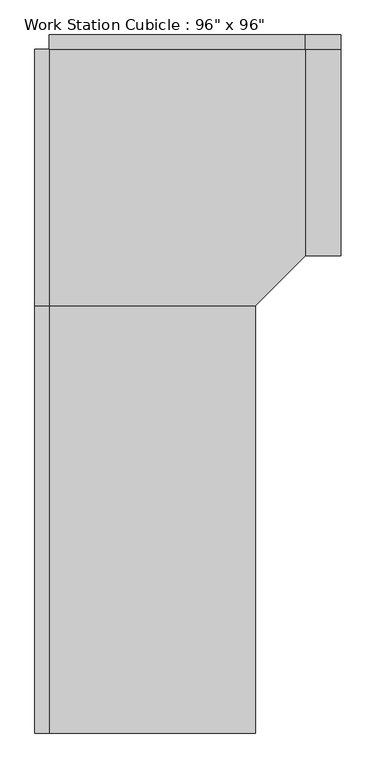
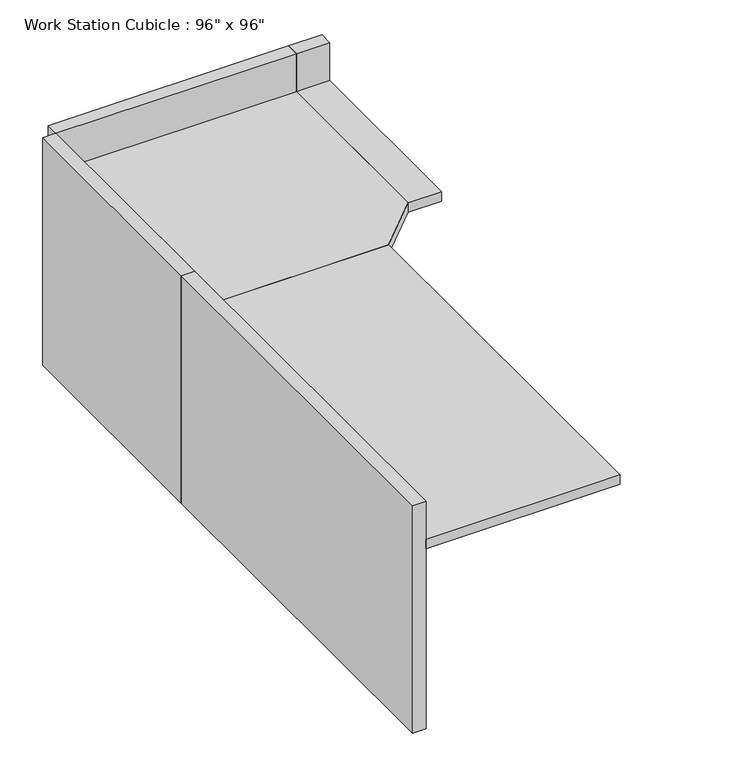
"""IFC4 building model written with IfcOpenShell, lengths in millimetres: furniture geometry."""

from ifc_helpers import new_model, si_unit, frame, origin, origin_with_axes, place, context, project, spatial, polyline, outline, extrude, source, transform, mapped, element, save


def furniture_6e13c3ce(model_context):
    return source(origin(), model_context, "Body", "SweptSolid", [
        extrude(outline(polyline([(-80.9317522, -545.8230076), (833.4682478, -545.8230076), (833.4682478, -1282.4230076), (655.6682478, -1460.2230076), (-80.9317522, -1460.2230076), (-80.9317522, -545.8230076)])), frame((0.0, 0.0, 723.9), z_axis=(0.0, 0.0, 1.0), x_axis=(1.0, 0.0, 0.0)), (0.0, 0.0, 1.0), 38.1),
        extrude(outline(polyline([(655.6682478, -2984.2230076), (-80.9317522, -2984.2230076), (-80.9317522, -1460.2230076), (655.6682478, -1460.2230076), (655.6682478, -2984.2230076)])), frame((0.0, 0.0, 723.9), z_axis=(0.0, 0.0, 1.0), x_axis=(1.0, 0.0, 0.0)), (0.0, 0.0, 1.0), 38.1),
        extrude(outline(polyline([(960.4682478, -1282.4230076), (833.4682478, -1282.4230076), (833.4682478, -545.8230076), (960.4682478, -545.8230076), (960.4682478, -1282.4230076)])), frame((0.0, 0.0, 723.9), z_axis=(0.0, 0.0, 1.0), x_axis=(1.0, 0.0, 0.0)), (0.0, 0.0, 1.0), 38.1),
        extrude(outline(polyline([(960.4682478, -545.8230076), (833.4682478, -545.8230076), (833.4682478, -495.0230076), (960.4682478, -495.0230076), (960.4682478, -545.8230076)])), origin_with_axes(), (0.0, 0.0, 1.0), 914.4),
        extrude(outline(polyline([(833.4682478, -545.8230076), (-80.9317522, -545.8230076), (-80.9317522, -495.0230076), (833.4682478, -495.0230076), (833.4682478, -545.8230076)])), origin_with_axes(), (0.0, 0.0, 1.0), 914.4),
        extrude(outline(polyline([(-80.9317522, -1460.2230076), (-131.7317522, -1460.2230076), (-131.7317522, -545.8230076), (-80.9317522, -545.8230076), (-80.9317522, -1460.2230076)])), origin_with_axes(), (0.0, 0.0, 1.0), 914.4),
        extrude(outline(polyline([(-80.9317522, -2984.2230076), (-131.7317522, -2984.2230076), (-131.7317522, -1460.2230076), (-80.9317522, -1460.2230076), (-80.9317522, -2984.2230076)])), origin_with_axes(), (0.0, 0.0, 1.0), 914.4),
    ])


if __name__ == "__main__":
    model = new_model("IFC4")
    model_context = context("Model", 3, world=origin())
    ifc_project = project(units=[si_unit("LENGTHUNIT", "METRE", prefix="MILLI")], contexts=[model_context])
    site = spatial("IfcSite", under=ifc_project)
    building = spatial("IfcBuilding", under=site)
    placement = place(None, origin())
    furniture_shape = furniture_6e13c3ce(model_context)
    element("IfcFurniture", 1, ObjectType="Work Station Cubicle : 96\" x 96\"", at=placement, inside=building, context=model_context, shape_type="MappedRepresentation", body=[
        mapped(furniture_shape, transform((0.0, 0.0, 0.0), x_axis=(1.0, 0.0, 0.0), y_axis=(0.0, 1.0, 0.0), z_axis=(0.0, 0.0, 1.0))),
    ])
    save(model, "model.ifc")

# Revit data of these elements
# Type "Work Station Cubicle : 96\" x 96\""
#   Assembly Code = "E2020"
#   Desktop Height = 2' - 6"
#   Desktop1 Width = 2' - 5"
#   Desktop2 Width = 2' - 5"
#   Panel Height = 3' - 0"
#   Panel1 Length = 5' - 0"
#   Panel2 Length = 0' - 5"
#   Cube Panel Material = Textile - Light Gray
#   Work Top Material = Laminate, Ivory, Matte
#   Default Elevation = 0
# Element 1 (IfcFurniture, "Work Station Cubicle : 96\" x 96\"")
#   Materials on its faces: "Textile - Light Gray", "Laminate, Ivory, Matte"
# Materials
#   "Textile - Light Gray": class "Fabric", colour RGB 204 204 204, transparency 0
#   "Laminate, Ivory, Matte": class "Plastic", colour RGB 247 247 239, transparency 0, Description = "Plastic Laminate - Ivory, Matte", Cost = 0
